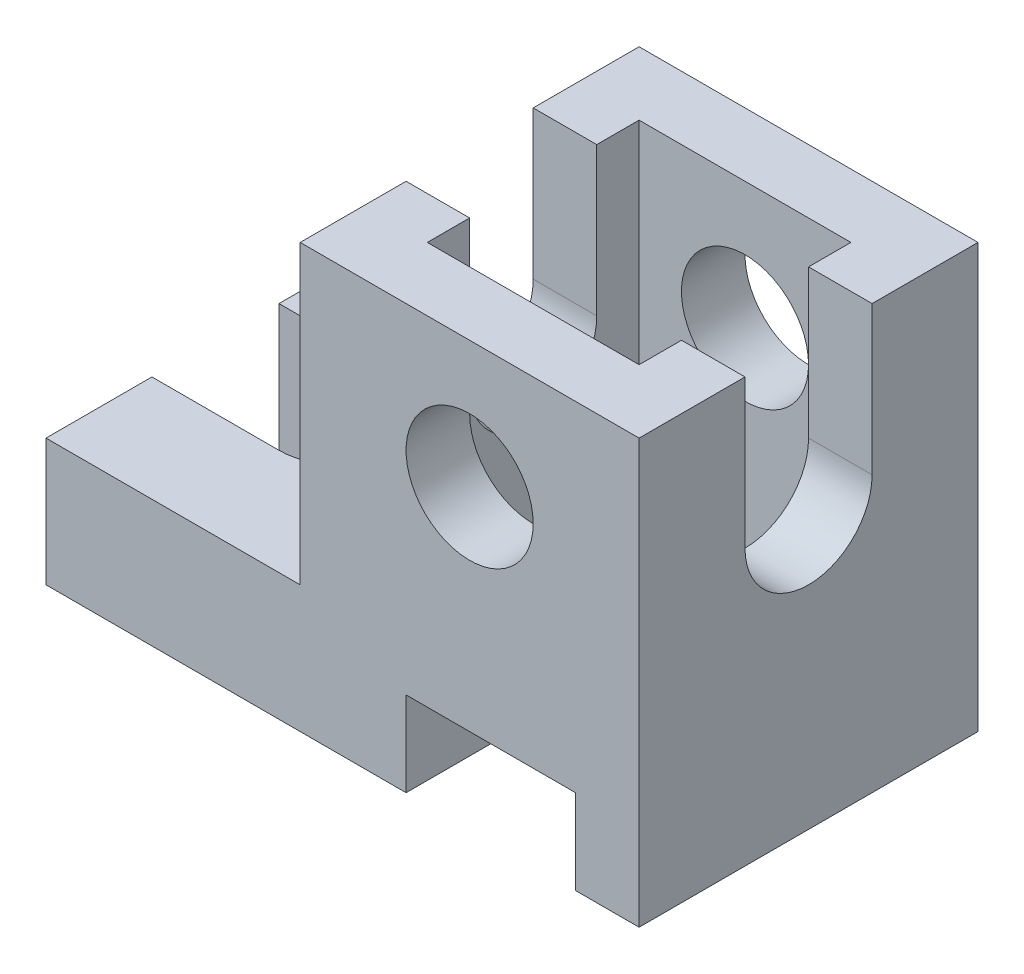
ISO-10303-21;
HEADER;
FILE_DESCRIPTION(('STEP AP214'),'2;1');
FILE_NAME('part.step','',(''),(''),'','','');
FILE_SCHEMA(('AUTOMOTIVE_DESIGN { 1 0 10303 214 1 1 1 1 }'));
ENDSEC;
DATA;
#1=APPLICATION_CONTEXT('core data for automotive mechanical design processes');
#2=APPLICATION_PROTOCOL_DEFINITION('international standard','automotive_design',2000,#1);
#3=PRODUCT_CONTEXT('',#1,'mechanical');
#4=PRODUCT('Part','Part','',(#3));
#5=PRODUCT_RELATED_PRODUCT_CATEGORY('part','',(#4));
#6=PRODUCT_DEFINITION_FORMATION('','',#4);
#7=PRODUCT_DEFINITION_CONTEXT('part definition',#1,'design');
#8=PRODUCT_DEFINITION('design','',#6,#7);
#9=PRODUCT_DEFINITION_SHAPE('','',#8);
#10=(LENGTH_UNIT() NAMED_UNIT(*) SI_UNIT(.MILLI.,.METRE.));
#11=(NAMED_UNIT(*) PLANE_ANGLE_UNIT() SI_UNIT($,.RADIAN.));
#12=(NAMED_UNIT(*) SI_UNIT($,.STERADIAN.) SOLID_ANGLE_UNIT());
#13=UNCERTAINTY_MEASURE_WITH_UNIT(LENGTH_MEASURE(1.E-05),#10,'distance_accuracy_value','');
#14=(GEOMETRIC_REPRESENTATION_CONTEXT(3) GLOBAL_UNCERTAINTY_ASSIGNED_CONTEXT((#13)) GLOBAL_UNIT_ASSIGNED_CONTEXT((#10,
#11,#12)) REPRESENTATION_CONTEXT('',''));
#15=CARTESIAN_POINT('',(0.,0.,0.));
#16=DIRECTION('',(0.,0.,1.));
#17=DIRECTION('',(1.,0.,0.));
#18=AXIS2_PLACEMENT_3D('',#15,#16,#17);
#19=CARTESIAN_POINT('',(140.,0.,-80.));
#20=DIRECTION('',(0.,-1.,0.));
#21=DIRECTION('',(0.,0.,-1.));
#22=AXIS2_PLACEMENT_3D('',#19,#20,#21);
#23=PLANE('',#22);
#24=DIRECTION('',(0.,0.,1.));
#25=VECTOR('',#24,1.);
#26=CARTESIAN_POINT('',(0.,0.,-80.));
#27=LINE('',#26,#25);
#28=CARTESIAN_POINT('',(0.,0.,-25.));
#29=VERTEX_POINT('',#28);
#30=CARTESIAN_POINT('',(0.,0.,0.));
#31=VERTEX_POINT('',#30);
#32=EDGE_CURVE('E244',#29,#31,#27,.T.);
#33=ORIENTED_EDGE('',*,*,#32,.F.);
#34=DIRECTION('',(1.,0.,0.));
#35=VECTOR('',#34,1.);
#36=CARTESIAN_POINT('',(140.,0.,-25.));
#37=LINE('',#36,#35);
#38=CARTESIAN_POINT('',(30.,0.,-25.));
#39=VERTEX_POINT('',#38);
#40=EDGE_CURVE('E285',#29,#39,#37,.T.);
#41=ORIENTED_EDGE('',*,*,#40,.T.);
#42=CARTESIAN_POINT('',(30.,0.,-40.));
#43=DIRECTION('',(0.,-1.,0.));
#44=DIRECTION('',(0.,0.,-1.));
#45=AXIS2_PLACEMENT_3D('',#42,#43,#44);
#46=CIRCLE('',#45,15.);
#47=CARTESIAN_POINT('',(30.,0.,-55.));
#48=VERTEX_POINT('',#47);
#49=EDGE_CURVE('E272',#39,#48,#46,.F.);
#50=ORIENTED_EDGE('',*,*,#49,.T.);
#51=DIRECTION('',(-1.,0.,0.));
#52=VECTOR('',#51,1.);
#53=CARTESIAN_POINT('',(140.,0.,-55.));
#54=LINE('',#53,#52);
#55=CARTESIAN_POINT('',(0.,0.,-55.));
#56=VERTEX_POINT('',#55);
#57=EDGE_CURVE('E277',#48,#56,#54,.T.);
#58=ORIENTED_EDGE('',*,*,#57,.T.);
#59=CARTESIAN_POINT('',(0.,0.,-80.));
#60=VERTEX_POINT('',#59);
#61=EDGE_CURVE('E239',#60,#56,#27,.T.);
#62=ORIENTED_EDGE('',*,*,#61,.F.);
#63=DIRECTION('',(1.,0.,0.));
#64=VECTOR('',#63,1.);
#65=CARTESIAN_POINT('',(140.,0.,-80.));
#66=LINE('',#65,#64);
#67=CARTESIAN_POINT('',(85.,0.,-80.));
#68=VERTEX_POINT('',#67);
#69=EDGE_CURVE('E420',#60,#68,#66,.T.);
#70=ORIENTED_EDGE('',*,*,#69,.T.);
#71=DIRECTION('',(0.,0.,1.));
#72=VECTOR('',#71,1.);
#73=CARTESIAN_POINT('',(85.,0.,-80.));
#74=LINE('',#73,#72);
#75=CARTESIAN_POINT('',(85.,0.,0.));
#76=VERTEX_POINT('',#75);
#77=EDGE_CURVE('E408',#68,#76,#74,.T.);
#78=ORIENTED_EDGE('',*,*,#77,.T.);
#79=DIRECTION('',(1.,0.,0.));
#80=VECTOR('',#79,1.);
#81=CARTESIAN_POINT('',(140.,0.,0.));
#82=LINE('',#81,#80);
#83=EDGE_CURVE('E430',#31,#76,#82,.T.);
#84=ORIENTED_EDGE('',*,*,#83,.F.);
#85=EDGE_LOOP('',(#33,#41,#50,#58,#62,#70,#78,#84));
#86=FACE_BOUND('',#85,.T.);
#87=ADVANCED_FACE('F44',(#86),#23,.T.);
#88=CARTESIAN_POINT('',(0.,0.,-80.));
#89=DIRECTION('',(-1.,0.,0.));
#90=DIRECTION('',(0.,0.,1.));
#91=AXIS2_PLACEMENT_3D('',#88,#89,#90);
#92=PLANE('',#91);
#93=DIRECTION('',(0.,0.,1.));
#94=VECTOR('',#93,1.);
#95=CARTESIAN_POINT('',(0.,30.,-80.));
#96=LINE('',#95,#94);
#97=CARTESIAN_POINT('',(0.,30.,-25.));
#98=VERTEX_POINT('',#97);
#99=CARTESIAN_POINT('',(0.,30.,0.));
#100=VERTEX_POINT('',#99);
#101=EDGE_CURVE('E247',#98,#100,#96,.T.);
#102=ORIENTED_EDGE('',*,*,#101,.F.);
#103=DIRECTION('',(0.,-1.,0.));
#104=VECTOR('',#103,1.);
#105=CARTESIAN_POINT('',(0.,40.,-25.));
#106=LINE('',#105,#104);
#107=EDGE_CURVE('E238',#98,#29,#106,.T.);
#108=ORIENTED_EDGE('',*,*,#107,.T.);
#109=ORIENTED_EDGE('',*,*,#32,.T.);
#110=DIRECTION('',(0.,-1.,0.));
#111=VECTOR('',#110,1.);
#112=CARTESIAN_POINT('',(0.,0.,0.));
#113=LINE('',#112,#111);
#114=EDGE_CURVE('E434',#100,#31,#113,.T.);
#115=ORIENTED_EDGE('',*,*,#114,.F.);
#116=EDGE_LOOP('',(#102,#108,#109,#115));
#117=FACE_BOUND('',#116,.T.);
#118=ADVANCED_FACE('F484',(#117),#92,.T.);
#119=ORIENTED_EDGE('',*,*,#61,.T.);
#120=DIRECTION('',(0.,-1.,0.));
#121=VECTOR('',#120,1.);
#122=CARTESIAN_POINT('',(0.,40.,-55.));
#123=LINE('',#122,#121);
#124=CARTESIAN_POINT('',(0.,30.,-55.));
#125=VERTEX_POINT('',#124);
#126=EDGE_CURVE('E223',#125,#56,#123,.T.);
#127=ORIENTED_EDGE('',*,*,#126,.F.);
#128=CARTESIAN_POINT('',(0.,30.,-80.));
#129=VERTEX_POINT('',#128);
#130=EDGE_CURVE('E240',#129,#125,#96,.T.);
#131=ORIENTED_EDGE('',*,*,#130,.F.);
#132=DIRECTION('',(0.,-1.,0.));
#133=VECTOR('',#132,1.);
#134=CARTESIAN_POINT('',(0.,0.,-80.));
#135=LINE('',#134,#133);
#136=EDGE_CURVE('E255',#129,#60,#135,.T.);
#137=ORIENTED_EDGE('',*,*,#136,.T.);
#138=EDGE_LOOP('',(#119,#127,#131,#137));
#139=FACE_BOUND('',#138,.T.);
#140=ADVANCED_FACE('F233',(#139),#92,.T.);
#141=CARTESIAN_POINT('',(0.,30.,-80.));
#142=DIRECTION('',(0.,1.,0.));
#143=DIRECTION('',(0.,0.,1.));
#144=AXIS2_PLACEMENT_3D('',#141,#142,#143);
#145=PLANE('',#144);
#146=CARTESIAN_POINT('',(30.,30.,-40.));
#147=DIRECTION('',(0.,1.,0.));
#148=DIRECTION('',(0.,0.,1.));
#149=AXIS2_PLACEMENT_3D('',#146,#147,#148);
#150=CIRCLE('',#149,15.);
#151=CARTESIAN_POINT('',(30.,30.,-55.));
#152=VERTEX_POINT('',#151);
#153=CARTESIAN_POINT('',(30.,30.,-25.));
#154=VERTEX_POINT('',#153);
#155=EDGE_CURVE('E52',#152,#154,#150,.F.);
#156=ORIENTED_EDGE('',*,*,#155,.T.);
#157=DIRECTION('',(-1.,0.,0.));
#158=VECTOR('',#157,1.);
#159=CARTESIAN_POINT('',(0.,30.,-25.));
#160=LINE('',#159,#158);
#161=EDGE_CURVE('E11',#154,#98,#160,.T.);
#162=ORIENTED_EDGE('',*,*,#161,.T.);
#163=ORIENTED_EDGE('',*,*,#101,.T.);
#164=DIRECTION('',(-1.,0.,0.));
#165=VECTOR('',#164,1.);
#166=CARTESIAN_POINT('',(0.,30.,0.));
#167=LINE('',#166,#165);
#168=CARTESIAN_POINT('',(60.,30.,0.));
#169=VERTEX_POINT('',#168);
#170=EDGE_CURVE('E433',#169,#100,#167,.T.);
#171=ORIENTED_EDGE('',*,*,#170,.F.);
#172=DIRECTION('',(0.,0.,1.));
#173=VECTOR('',#172,1.);
#174=CARTESIAN_POINT('',(60.,30.,-80.));
#175=LINE('',#174,#173);
#176=CARTESIAN_POINT('',(60.,30.,-80.));
#177=VERTEX_POINT('',#176);
#178=EDGE_CURVE('E378',#177,#169,#175,.T.);
#179=ORIENTED_EDGE('',*,*,#178,.F.);
#180=DIRECTION('',(-1.,0.,0.));
#181=VECTOR('',#180,1.);
#182=CARTESIAN_POINT('',(0.,30.,-80.));
#183=LINE('',#182,#181);
#184=EDGE_CURVE('E242',#177,#129,#183,.T.);
#185=ORIENTED_EDGE('',*,*,#184,.T.);
#186=ORIENTED_EDGE('',*,*,#130,.T.);
#187=DIRECTION('',(1.,0.,0.));
#188=VECTOR('',#187,1.);
#189=CARTESIAN_POINT('',(0.,30.,-55.));
#190=LINE('',#189,#188);
#191=EDGE_CURVE('E225',#125,#152,#190,.T.);
#192=ORIENTED_EDGE('',*,*,#191,.T.);
#193=EDGE_LOOP('',(#156,#162,#163,#171,#179,#185,#186,#192));
#194=FACE_BOUND('',#193,.T.);
#195=ADVANCED_FACE('F245',(#194),#145,.T.);
#196=CARTESIAN_POINT('',(140.,100.,-80.));
#197=DIRECTION('',(0.,1.,0.));
#198=DIRECTION('',(0.,0.,1.));
#199=AXIS2_PLACEMENT_3D('',#196,#197,#198);
#200=PLANE('',#199);
#201=DIRECTION('',(0.,0.,1.));
#202=VECTOR('',#201,1.);
#203=CARTESIAN_POINT('',(60.,100.,-80.));
#204=LINE('',#203,#202);
#205=CARTESIAN_POINT('',(60.,100.,-80.));
#206=VERTEX_POINT('',#205);
#207=CARTESIAN_POINT('',(60.,100.,-55.));
#208=VERTEX_POINT('',#207);
#209=EDGE_CURVE('E385',#206,#208,#204,.T.);
#210=ORIENTED_EDGE('',*,*,#209,.T.);
#211=DIRECTION('',(-1.,0.,0.));
#212=VECTOR('',#211,1.);
#213=CARTESIAN_POINT('',(140.,100.,-55.));
#214=LINE('',#213,#212);
#215=CARTESIAN_POINT('',(75.,100.,-55.));
#216=VERTEX_POINT('',#215);
#217=EDGE_CURVE('E301',#216,#208,#214,.T.);
#218=ORIENTED_EDGE('',*,*,#217,.F.);
#219=DIRECTION('',(0.,0.,-1.));
#220=VECTOR('',#219,1.);
#221=CARTESIAN_POINT('',(75.,100.,0.));
#222=LINE('',#221,#220);
#223=CARTESIAN_POINT('',(75.,100.,-65.));
#224=VERTEX_POINT('',#223);
#225=EDGE_CURVE('E330',#216,#224,#222,.T.);
#226=ORIENTED_EDGE('',*,*,#225,.T.);
#227=DIRECTION('',(1.,0.,0.));
#228=VECTOR('',#227,1.);
#229=CARTESIAN_POINT('',(0.,100.,-65.));
#230=LINE('',#229,#228);
#231=CARTESIAN_POINT('',(125.,100.,-65.));
#232=VERTEX_POINT('',#231);
#233=EDGE_CURVE('E335',#224,#232,#230,.T.);
#234=ORIENTED_EDGE('',*,*,#233,.T.);
#235=DIRECTION('',(0.,0.,1.));
#236=VECTOR('',#235,1.);
#237=CARTESIAN_POINT('',(125.,100.,0.));
#238=LINE('',#237,#236);
#239=CARTESIAN_POINT('',(125.,100.,-55.));
#240=VERTEX_POINT('',#239);
#241=EDGE_CURVE('E346',#232,#240,#238,.T.);
#242=ORIENTED_EDGE('',*,*,#241,.T.);
#243=CARTESIAN_POINT('',(140.,100.,-55.));
#244=VERTEX_POINT('',#243);
#245=EDGE_CURVE('E302',#244,#240,#214,.T.);
#246=ORIENTED_EDGE('',*,*,#245,.F.);
#247=DIRECTION('',(0.,0.,1.));
#248=VECTOR('',#247,1.);
#249=CARTESIAN_POINT('',(140.,100.,-80.));
#250=LINE('',#249,#248);
#251=CARTESIAN_POINT('',(140.,100.,-80.));
#252=VERTEX_POINT('',#251);
#253=EDGE_CURVE('E387',#252,#244,#250,.T.);
#254=ORIENTED_EDGE('',*,*,#253,.F.);
#255=DIRECTION('',(-1.,0.,0.));
#256=VECTOR('',#255,1.);
#257=CARTESIAN_POINT('',(140.,100.,-80.));
#258=LINE('',#257,#256);
#259=EDGE_CURVE('E368',#252,#206,#258,.T.);
#260=ORIENTED_EDGE('',*,*,#259,.T.);
#261=EDGE_LOOP('',(#210,#218,#226,#234,#242,#246,#254,#260));
#262=FACE_BOUND('',#261,.T.);
#263=ADVANCED_FACE('F451',(#262),#200,.T.);
#264=CARTESIAN_POINT('',(140.,100.,-25.));
#265=VERTEX_POINT('',#264);
#266=CARTESIAN_POINT('',(140.,100.,0.));
#267=VERTEX_POINT('',#266);
#268=EDGE_CURVE('E373',#265,#267,#250,.T.);
#269=ORIENTED_EDGE('',*,*,#268,.F.);
#270=DIRECTION('',(-1.,0.,0.));
#271=VECTOR('',#270,1.);
#272=CARTESIAN_POINT('',(140.,100.,-25.));
#273=LINE('',#272,#271);
#274=CARTESIAN_POINT('',(125.,100.,-25.));
#275=VERTEX_POINT('',#274);
#276=EDGE_CURVE('E303',#265,#275,#273,.T.);
#277=ORIENTED_EDGE('',*,*,#276,.T.);
#278=CARTESIAN_POINT('',(125.,100.,-15.));
#279=VERTEX_POINT('',#278);
#280=EDGE_CURVE('E350',#275,#279,#238,.T.);
#281=ORIENTED_EDGE('',*,*,#280,.T.);
#282=DIRECTION('',(-1.,0.,0.));
#283=VECTOR('',#282,1.);
#284=CARTESIAN_POINT('',(0.,100.,-15.));
#285=LINE('',#284,#283);
#286=CARTESIAN_POINT('',(75.,100.,-15.));
#287=VERTEX_POINT('',#286);
#288=EDGE_CURVE('E341',#279,#287,#285,.T.);
#289=ORIENTED_EDGE('',*,*,#288,.T.);
#290=CARTESIAN_POINT('',(75.,100.,-25.));
#291=VERTEX_POINT('',#290);
#292=EDGE_CURVE('E342',#287,#291,#222,.T.);
#293=ORIENTED_EDGE('',*,*,#292,.T.);
#294=CARTESIAN_POINT('',(60.,100.,-25.));
#295=VERTEX_POINT('',#294);
#296=EDGE_CURVE('E306',#291,#295,#273,.T.);
#297=ORIENTED_EDGE('',*,*,#296,.T.);
#298=CARTESIAN_POINT('',(60.,100.,0.));
#299=VERTEX_POINT('',#298);
#300=EDGE_CURVE('E384',#295,#299,#204,.T.);
#301=ORIENTED_EDGE('',*,*,#300,.T.);
#302=DIRECTION('',(-1.,0.,0.));
#303=VECTOR('',#302,1.);
#304=CARTESIAN_POINT('',(140.,100.,0.));
#305=LINE('',#304,#303);
#306=EDGE_CURVE('E364',#267,#299,#305,.T.);
#307=ORIENTED_EDGE('',*,*,#306,.F.);
#308=EDGE_LOOP('',(#269,#277,#281,#289,#293,#297,#301,#307));
#309=FACE_BOUND('',#308,.T.);
#310=ADVANCED_FACE('F475',(#309),#200,.T.);
#311=CARTESIAN_POINT('',(140.,30.,-80.));
#312=DIRECTION('',(1.,0.,0.));
#313=DIRECTION('',(0.,0.,-1.));
#314=AXIS2_PLACEMENT_3D('',#311,#312,#313);
#315=PLANE('',#314);
#316=ORIENTED_EDGE('',*,*,#253,.T.);
#317=DIRECTION('',(0.,1.,0.));
#318=VECTOR('',#317,1.);
#319=CARTESIAN_POINT('',(140.,0.,-55.));
#320=LINE('',#319,#318);
#321=CARTESIAN_POINT('',(140.,65.,-55.));
#322=VERTEX_POINT('',#321);
#323=EDGE_CURVE('E284',#322,#244,#320,.T.);
#324=ORIENTED_EDGE('',*,*,#323,.F.);
#325=CARTESIAN_POINT('',(140.,65.,-40.));
#326=DIRECTION('',(-1.,0.,0.));
#327=DIRECTION('',(0.,0.,1.));
#328=AXIS2_PLACEMENT_3D('',#325,#326,#327);
#329=CIRCLE('',#328,15.);
#330=CARTESIAN_POINT('',(140.,65.,-25.));
#331=VERTEX_POINT('',#330);
#332=EDGE_CURVE('E289',#322,#331,#329,.T.);
#333=ORIENTED_EDGE('',*,*,#332,.T.);
#334=DIRECTION('',(0.,-1.,0.));
#335=VECTOR('',#334,1.);
#336=CARTESIAN_POINT('',(140.,0.,-25.));
#337=LINE('',#336,#335);
#338=EDGE_CURVE('E292',#265,#331,#337,.T.);
#339=ORIENTED_EDGE('',*,*,#338,.F.);
#340=ORIENTED_EDGE('',*,*,#268,.T.);
#341=DIRECTION('',(0.,1.,0.));
#342=VECTOR('',#341,1.);
#343=CARTESIAN_POINT('',(140.,30.,0.));
#344=LINE('',#343,#342);
#345=CARTESIAN_POINT('',(140.,0.,0.));
#346=VERTEX_POINT('',#345);
#347=EDGE_CURVE('E429',#346,#267,#344,.T.);
#348=ORIENTED_EDGE('',*,*,#347,.F.);
#349=DIRECTION('',(0.,0.,1.));
#350=VECTOR('',#349,1.);
#351=CARTESIAN_POINT('',(140.,0.,-80.));
#352=LINE('',#351,#350);
#353=CARTESIAN_POINT('',(140.,0.,-80.));
#354=VERTEX_POINT('',#353);
#355=EDGE_CURVE('E246',#354,#346,#352,.T.);
#356=ORIENTED_EDGE('',*,*,#355,.F.);
#357=DIRECTION('',(0.,1.,0.));
#358=VECTOR('',#357,1.);
#359=CARTESIAN_POINT('',(140.,30.,-80.));
#360=LINE('',#359,#358);
#361=EDGE_CURVE('E425',#354,#252,#360,.T.);
#362=ORIENTED_EDGE('',*,*,#361,.T.);
#363=EDGE_LOOP('',(#316,#324,#333,#339,#340,#348,#356,#362));
#364=FACE_BOUND('',#363,.T.);
#365=ADVANCED_FACE('F446',(#364),#315,.T.);
#366=CARTESIAN_POINT('',(125.,0.,-80.));
#367=DIRECTION('',(1.,0.,0.));
#368=DIRECTION('',(0.,0.,-1.));
#369=AXIS2_PLACEMENT_3D('',#366,#367,#368);
#370=PLANE('',#369);
#371=DIRECTION('',(0.,-1.,0.));
#372=VECTOR('',#371,1.);
#373=CARTESIAN_POINT('',(125.,0.,-55.));
#374=LINE('',#373,#372);
#375=CARTESIAN_POINT('',(125.,65.,-55.));
#376=VERTEX_POINT('',#375);
#377=EDGE_CURVE('E318',#240,#376,#374,.T.);
#378=ORIENTED_EDGE('',*,*,#377,.F.);
#379=ORIENTED_EDGE('',*,*,#241,.F.);
#380=DIRECTION('',(0.,1.,0.));
#381=VECTOR('',#380,1.);
#382=CARTESIAN_POINT('',(125.,20.,-65.));
#383=LINE('',#382,#381);
#384=CARTESIAN_POINT('',(125.,20.,-65.));
#385=VERTEX_POINT('',#384);
#386=EDGE_CURVE('E359',#385,#232,#383,.T.);
#387=ORIENTED_EDGE('',*,*,#386,.F.);
#388=DIRECTION('',(0.,0.,1.));
#389=VECTOR('',#388,1.);
#390=CARTESIAN_POINT('',(125.,20.,-80.));
#391=LINE('',#390,#389);
#392=CARTESIAN_POINT('',(125.,20.,-80.));
#393=VERTEX_POINT('',#392);
#394=EDGE_CURVE('E411',#393,#385,#391,.T.);
#395=ORIENTED_EDGE('',*,*,#394,.F.);
#396=DIRECTION('',(0.,1.,0.));
#397=VECTOR('',#396,1.);
#398=CARTESIAN_POINT('',(125.,0.,-80.));
#399=LINE('',#398,#397);
#400=CARTESIAN_POINT('',(125.,0.,-80.));
#401=VERTEX_POINT('',#400);
#402=EDGE_CURVE('E386',#401,#393,#399,.T.);
#403=ORIENTED_EDGE('',*,*,#402,.F.);
#404=DIRECTION('',(0.,0.,1.));
#405=VECTOR('',#404,1.);
#406=CARTESIAN_POINT('',(125.,0.,-80.));
#407=LINE('',#406,#405);
#408=CARTESIAN_POINT('',(125.,0.,0.));
#409=VERTEX_POINT('',#408);
#410=EDGE_CURVE('E396',#401,#409,#407,.T.);
#411=ORIENTED_EDGE('',*,*,#410,.T.);
#412=DIRECTION('',(0.,1.,0.));
#413=VECTOR('',#412,1.);
#414=CARTESIAN_POINT('',(125.,0.,0.));
#415=LINE('',#414,#413);
#416=CARTESIAN_POINT('',(125.,20.,0.));
#417=VERTEX_POINT('',#416);
#418=EDGE_CURVE('E381',#409,#417,#415,.T.);
#419=ORIENTED_EDGE('',*,*,#418,.T.);
#420=CARTESIAN_POINT('',(125.,20.,-15.));
#421=VERTEX_POINT('',#420);
#422=EDGE_CURVE('E417',#421,#417,#391,.T.);
#423=ORIENTED_EDGE('',*,*,#422,.F.);
#424=DIRECTION('',(0.,1.,0.));
#425=VECTOR('',#424,1.);
#426=CARTESIAN_POINT('',(125.,20.,-15.));
#427=LINE('',#426,#425);
#428=EDGE_CURVE('E356',#421,#279,#427,.T.);
#429=ORIENTED_EDGE('',*,*,#428,.T.);
#430=ORIENTED_EDGE('',*,*,#280,.F.);
#431=DIRECTION('',(0.,1.,0.));
#432=VECTOR('',#431,1.);
#433=CARTESIAN_POINT('',(125.,0.,-25.));
#434=LINE('',#433,#432);
#435=CARTESIAN_POINT('',(125.,65.,-25.));
#436=VERTEX_POINT('',#435);
#437=EDGE_CURVE('E316',#436,#275,#434,.T.);
#438=ORIENTED_EDGE('',*,*,#437,.F.);
#439=CARTESIAN_POINT('',(125.,65.,-40.));
#440=DIRECTION('',(1.,0.,0.));
#441=DIRECTION('',(0.,0.,-1.));
#442=AXIS2_PLACEMENT_3D('',#439,#440,#441);
#443=CIRCLE('',#442,15.);
#444=EDGE_CURVE('E305',#436,#376,#443,.T.);
#445=ORIENTED_EDGE('',*,*,#444,.T.);
#446=EDGE_LOOP('',(#378,#379,#387,#395,#403,#411,#419,#423,#429,#430,#438,#445));
#447=FACE_BOUND('',#446,.T.);
#448=ADVANCED_FACE('F466',(#447),#370,.F.);
#449=CARTESIAN_POINT('',(60.,100.,-80.));
#450=DIRECTION('',(-1.,0.,0.));
#451=DIRECTION('',(0.,0.,1.));
#452=AXIS2_PLACEMENT_3D('',#449,#450,#451);
#453=PLANE('',#452);
#454=CARTESIAN_POINT('',(60.,65.,-40.));
#455=DIRECTION('',(-1.,0.,0.));
#456=DIRECTION('',(0.,0.,1.));
#457=AXIS2_PLACEMENT_3D('',#454,#455,#456);
#458=CIRCLE('',#457,15.);
#459=CARTESIAN_POINT('',(60.,65.,-55.));
#460=VERTEX_POINT('',#459);
#461=CARTESIAN_POINT('',(60.,65.,-25.));
#462=VERTEX_POINT('',#461);
#463=EDGE_CURVE('E298',#460,#462,#458,.T.);
#464=ORIENTED_EDGE('',*,*,#463,.F.);
#465=DIRECTION('',(0.,1.,0.));
#466=VECTOR('',#465,1.);
#467=CARTESIAN_POINT('',(60.,0.,-55.));
#468=LINE('',#467,#466);
#469=EDGE_CURVE('E282',#460,#208,#468,.T.);
#470=ORIENTED_EDGE('',*,*,#469,.T.);
#471=ORIENTED_EDGE('',*,*,#209,.F.);
#472=DIRECTION('',(0.,-1.,0.));
#473=VECTOR('',#472,1.);
#474=CARTESIAN_POINT('',(60.,100.,-80.));
#475=LINE('',#474,#473);
#476=EDGE_CURVE('E369',#206,#177,#475,.T.);
#477=ORIENTED_EDGE('',*,*,#476,.T.);
#478=ORIENTED_EDGE('',*,*,#178,.T.);
#479=DIRECTION('',(0.,-1.,0.));
#480=VECTOR('',#479,1.);
#481=CARTESIAN_POINT('',(60.,100.,0.));
#482=LINE('',#481,#480);
#483=EDGE_CURVE('E367',#299,#169,#482,.T.);
#484=ORIENTED_EDGE('',*,*,#483,.F.);
#485=ORIENTED_EDGE('',*,*,#300,.F.);
#486=DIRECTION('',(0.,-1.,0.));
#487=VECTOR('',#486,1.);
#488=CARTESIAN_POINT('',(60.,0.,-25.));
#489=LINE('',#488,#487);
#490=EDGE_CURVE('E290',#295,#462,#489,.T.);
#491=ORIENTED_EDGE('',*,*,#490,.T.);
#492=EDGE_LOOP('',(#464,#470,#471,#477,#478,#484,#485,#491));
#493=FACE_BOUND('',#492,.T.);
#494=ADVANCED_FACE('F483',(#493),#453,.T.);
#495=CARTESIAN_POINT('',(75.,20.,0.));
#496=DIRECTION('',(1.,0.,0.));
#497=DIRECTION('',(0.,0.,-1.));
#498=AXIS2_PLACEMENT_3D('',#495,#496,#497);
#499=PLANE('',#498);
#500=ORIENTED_EDGE('',*,*,#225,.F.);
#501=DIRECTION('',(0.,-1.,0.));
#502=VECTOR('',#501,1.);
#503=CARTESIAN_POINT('',(75.,20.,-55.));
#504=LINE('',#503,#502);
#505=CARTESIAN_POINT('',(75.,65.,-55.));
#506=VERTEX_POINT('',#505);
#507=EDGE_CURVE('E229',#216,#506,#504,.T.);
#508=ORIENTED_EDGE('',*,*,#507,.T.);
#509=CARTESIAN_POINT('',(75.,65.,-40.));
#510=DIRECTION('',(1.,0.,0.));
#511=DIRECTION('',(0.,0.,-1.));
#512=AXIS2_PLACEMENT_3D('',#509,#510,#511);
#513=CIRCLE('',#512,15.);
#514=CARTESIAN_POINT('',(75.,65.,-25.));
#515=VERTEX_POINT('',#514);
#516=EDGE_CURVE('E257',#515,#506,#513,.T.);
#517=ORIENTED_EDGE('',*,*,#516,.F.);
#518=DIRECTION('',(0.,1.,0.));
#519=VECTOR('',#518,1.);
#520=CARTESIAN_POINT('',(75.,20.,-25.));
#521=LINE('',#520,#519);
#522=EDGE_CURVE('E265',#515,#291,#521,.T.);
#523=ORIENTED_EDGE('',*,*,#522,.T.);
#524=ORIENTED_EDGE('',*,*,#292,.F.);
#525=DIRECTION('',(0.,1.,0.));
#526=VECTOR('',#525,1.);
#527=CARTESIAN_POINT('',(75.,20.,-15.));
#528=LINE('',#527,#526);
#529=CARTESIAN_POINT('',(75.,20.,-15.));
#530=VERTEX_POINT('',#529);
#531=EDGE_CURVE('E339',#530,#287,#528,.T.);
#532=ORIENTED_EDGE('',*,*,#531,.F.);
#533=DIRECTION('',(0.,0.,-1.));
#534=VECTOR('',#533,1.);
#535=CARTESIAN_POINT('',(75.,20.,0.));
#536=LINE('',#535,#534);
#537=CARTESIAN_POINT('',(75.,20.,-65.));
#538=VERTEX_POINT('',#537);
#539=EDGE_CURVE('E327',#530,#538,#536,.T.);
#540=ORIENTED_EDGE('',*,*,#539,.T.);
#541=DIRECTION('',(0.,1.,0.));
#542=VECTOR('',#541,1.);
#543=CARTESIAN_POINT('',(75.,20.,-65.));
#544=LINE('',#543,#542);
#545=EDGE_CURVE('E351',#538,#224,#544,.T.);
#546=ORIENTED_EDGE('',*,*,#545,.T.);
#547=EDGE_LOOP('',(#500,#508,#517,#523,#524,#532,#540,#546));
#548=FACE_BOUND('',#547,.T.);
#549=ADVANCED_FACE('F520',(#548),#499,.T.);
#550=CARTESIAN_POINT('',(0.,20.,-80.));
#551=DIRECTION('',(0.,1.,0.));
#552=DIRECTION('',(0.,0.,1.));
#553=AXIS2_PLACEMENT_3D('',#550,#551,#552);
#554=PLANE('',#553);
#555=DIRECTION('',(1.,0.,0.));
#556=VECTOR('',#555,1.);
#557=CARTESIAN_POINT('',(0.,20.,-65.));
#558=LINE('',#557,#556);
#559=CARTESIAN_POINT('',(85.,20.,-65.));
#560=VERTEX_POINT('',#559);
#561=EDGE_CURVE('E338',#560,#385,#558,.T.);
#562=ORIENTED_EDGE('',*,*,#561,.F.);
#563=DIRECTION('',(0.,0.,1.));
#564=VECTOR('',#563,1.);
#565=CARTESIAN_POINT('',(85.,20.,-80.));
#566=LINE('',#565,#564);
#567=CARTESIAN_POINT('',(85.,20.,-80.));
#568=VERTEX_POINT('',#567);
#569=EDGE_CURVE('E409',#568,#560,#566,.T.);
#570=ORIENTED_EDGE('',*,*,#569,.F.);
#571=DIRECTION('',(-1.,0.,0.));
#572=VECTOR('',#571,1.);
#573=CARTESIAN_POINT('',(0.,20.,-80.));
#574=LINE('',#573,#572);
#575=EDGE_CURVE('E395',#393,#568,#574,.T.);
#576=ORIENTED_EDGE('',*,*,#575,.F.);
#577=ORIENTED_EDGE('',*,*,#394,.T.);
#578=EDGE_LOOP('',(#562,#570,#576,#577));
#579=FACE_BOUND('',#578,.T.);
#580=ADVANCED_FACE('F502',(#579),#554,.F.);
#581=DIRECTION('',(-1.,0.,0.));
#582=VECTOR('',#581,1.);
#583=CARTESIAN_POINT('',(0.,20.,-15.));
#584=LINE('',#583,#582);
#585=CARTESIAN_POINT('',(85.,20.,-15.));
#586=VERTEX_POINT('',#585);
#587=EDGE_CURVE('E334',#421,#586,#584,.T.);
#588=ORIENTED_EDGE('',*,*,#587,.F.);
#589=ORIENTED_EDGE('',*,*,#422,.T.);
#590=DIRECTION('',(-1.,0.,0.));
#591=VECTOR('',#590,1.);
#592=CARTESIAN_POINT('',(0.,20.,0.));
#593=LINE('',#592,#591);
#594=CARTESIAN_POINT('',(85.,20.,0.));
#595=VERTEX_POINT('',#594);
#596=EDGE_CURVE('E405',#417,#595,#593,.T.);
#597=ORIENTED_EDGE('',*,*,#596,.T.);
#598=EDGE_CURVE('E415',#586,#595,#566,.T.);
#599=ORIENTED_EDGE('',*,*,#598,.F.);
#600=EDGE_LOOP('',(#588,#589,#597,#599));
#601=FACE_BOUND('',#600,.T.);
#602=ADVANCED_FACE('F496',(#601),#554,.F.);
#603=ORIENTED_EDGE('',*,*,#410,.F.);
#604=EDGE_CURVE('E421',#401,#354,#66,.T.);
#605=ORIENTED_EDGE('',*,*,#604,.T.);
#606=ORIENTED_EDGE('',*,*,#355,.T.);
#607=EDGE_CURVE('E407',#409,#346,#82,.T.);
#608=ORIENTED_EDGE('',*,*,#607,.F.);
#609=EDGE_LOOP('',(#603,#605,#606,#608));
#610=FACE_BOUND('',#609,.T.);
#611=ADVANCED_FACE('F50',(#610),#23,.T.);
#612=CARTESIAN_POINT('',(0.,0.,-80.));
#613=DIRECTION('',(0.,0.,-1.));
#614=DIRECTION('',(-1.,0.,0.));
#615=AXIS2_PLACEMENT_3D('',#612,#613,#614);
#616=PLANE('',#615);
#617=CARTESIAN_POINT('',(100.,70.,-80.));
#618=DIRECTION('',(0.,0.,1.));
#619=DIRECTION('',(1.,0.,0.));
#620=AXIS2_PLACEMENT_3D('',#617,#618,#619);
#621=CIRCLE('',#620,15.);
#622=CARTESIAN_POINT('',(115.,70.,-80.));
#623=VERTEX_POINT('',#622);
#624=EDGE_CURVE('E259',#623,#623,#621,.T.);
#625=ORIENTED_EDGE('',*,*,#624,.T.);
#626=EDGE_LOOP('',(#625));
#627=FACE_BOUND('',#626,.T.);
#628=DIRECTION('',(0.,-1.,0.));
#629=VECTOR('',#628,1.);
#630=CARTESIAN_POINT('',(85.,0.,-80.));
#631=LINE('',#630,#629);
#632=EDGE_CURVE('E397',#568,#68,#631,.T.);
#633=ORIENTED_EDGE('',*,*,#632,.T.);
#634=ORIENTED_EDGE('',*,*,#69,.F.);
#635=ORIENTED_EDGE('',*,*,#136,.F.);
#636=ORIENTED_EDGE('',*,*,#184,.F.);
#637=ORIENTED_EDGE('',*,*,#476,.F.);
#638=ORIENTED_EDGE('',*,*,#259,.F.);
#639=ORIENTED_EDGE('',*,*,#361,.F.);
#640=ORIENTED_EDGE('',*,*,#604,.F.);
#641=ORIENTED_EDGE('',*,*,#402,.T.);
#642=ORIENTED_EDGE('',*,*,#575,.T.);
#643=EDGE_LOOP('',(#633,#634,#635,#636,#637,#638,#639,#640,#641,#642));
#644=FACE_BOUND('',#643,.T.);
#645=ADVANCED_FACE('F452',(#627,#644),#616,.T.);
#646=CARTESIAN_POINT('',(0.,0.,0.));
#647=DIRECTION('',(0.,0.,-1.));
#648=DIRECTION('',(-1.,0.,0.));
#649=AXIS2_PLACEMENT_3D('',#646,#647,#648);
#650=PLANE('',#649);
#651=CARTESIAN_POINT('',(100.,70.,0.));
#652=DIRECTION('',(0.,0.,1.));
#653=DIRECTION('',(1.,0.,0.));
#654=AXIS2_PLACEMENT_3D('',#651,#652,#653);
#655=CIRCLE('',#654,15.);
#656=CARTESIAN_POINT('',(115.,70.,0.));
#657=VERTEX_POINT('',#656);
#658=EDGE_CURVE('E319',#657,#657,#655,.T.);
#659=ORIENTED_EDGE('',*,*,#658,.F.);
#660=EDGE_LOOP('',(#659));
#661=FACE_BOUND('',#660,.T.);
#662=ORIENTED_EDGE('',*,*,#83,.T.);
#663=DIRECTION('',(0.,-1.,0.));
#664=VECTOR('',#663,1.);
#665=CARTESIAN_POINT('',(85.,0.,0.));
#666=LINE('',#665,#664);
#667=EDGE_CURVE('E391',#595,#76,#666,.T.);
#668=ORIENTED_EDGE('',*,*,#667,.F.);
#669=ORIENTED_EDGE('',*,*,#596,.F.);
#670=ORIENTED_EDGE('',*,*,#418,.F.);
#671=ORIENTED_EDGE('',*,*,#607,.T.);
#672=ORIENTED_EDGE('',*,*,#347,.T.);
#673=ORIENTED_EDGE('',*,*,#306,.T.);
#674=ORIENTED_EDGE('',*,*,#483,.T.);
#675=ORIENTED_EDGE('',*,*,#170,.T.);
#676=ORIENTED_EDGE('',*,*,#114,.T.);
#677=EDGE_LOOP('',(#662,#668,#669,#670,#671,#672,#673,#674,#675,#676));
#678=FACE_BOUND('',#677,.T.);
#679=ADVANCED_FACE('F478',(#661,#678),#650,.F.);
#680=CARTESIAN_POINT('',(85.,0.,-80.));
#681=DIRECTION('',(-1.,0.,0.));
#682=DIRECTION('',(0.,0.,1.));
#683=AXIS2_PLACEMENT_3D('',#680,#681,#682);
#684=PLANE('',#683);
#685=ORIENTED_EDGE('',*,*,#667,.T.);
#686=ORIENTED_EDGE('',*,*,#77,.F.);
#687=ORIENTED_EDGE('',*,*,#632,.F.);
#688=ORIENTED_EDGE('',*,*,#569,.T.);
#689=DIRECTION('',(0.,0.,-1.));
#690=VECTOR('',#689,1.);
#691=CARTESIAN_POINT('',(85.,20.,-80.));
#692=LINE('',#691,#690);
#693=EDGE_CURVE('E357',#586,#560,#692,.T.);
#694=ORIENTED_EDGE('',*,*,#693,.F.);
#695=ORIENTED_EDGE('',*,*,#598,.T.);
#696=EDGE_LOOP('',(#685,#686,#687,#688,#694,#695));
#697=FACE_BOUND('',#696,.T.);
#698=ADVANCED_FACE('F492',(#697),#684,.F.);
#699=CARTESIAN_POINT('',(0.,20.,0.));
#700=DIRECTION('',(0.,1.,0.));
#701=DIRECTION('',(0.,0.,1.));
#702=AXIS2_PLACEMENT_3D('',#699,#700,#701);
#703=PLANE('',#702);
#704=ORIENTED_EDGE('',*,*,#693,.T.);
#705=EDGE_CURVE('E340',#538,#560,#558,.T.);
#706=ORIENTED_EDGE('',*,*,#705,.F.);
#707=ORIENTED_EDGE('',*,*,#539,.F.);
#708=EDGE_CURVE('E332',#586,#530,#584,.T.);
#709=ORIENTED_EDGE('',*,*,#708,.F.);
#710=EDGE_LOOP('',(#704,#706,#707,#709));
#711=FACE_BOUND('',#710,.T.);
#712=ADVANCED_FACE('F511',(#711),#703,.T.);
#713=CARTESIAN_POINT('',(0.,20.,-65.));
#714=DIRECTION('',(0.,0.,1.));
#715=DIRECTION('',(1.,0.,0.));
#716=AXIS2_PLACEMENT_3D('',#713,#714,#715);
#717=PLANE('',#716);
#718=CARTESIAN_POINT('',(100.,70.,-65.));
#719=DIRECTION('',(0.,0.,1.));
#720=DIRECTION('',(1.,0.,0.));
#721=AXIS2_PLACEMENT_3D('',#718,#719,#720);
#722=CIRCLE('',#721,15.);
#723=CARTESIAN_POINT('',(115.,70.,-65.));
#724=VERTEX_POINT('',#723);
#725=EDGE_CURVE('E256',#724,#724,#722,.T.);
#726=ORIENTED_EDGE('',*,*,#725,.F.);
#727=EDGE_LOOP('',(#726));
#728=FACE_BOUND('',#727,.T.);
#729=ORIENTED_EDGE('',*,*,#233,.F.);
#730=ORIENTED_EDGE('',*,*,#545,.F.);
#731=ORIENTED_EDGE('',*,*,#705,.T.);
#732=ORIENTED_EDGE('',*,*,#561,.T.);
#733=ORIENTED_EDGE('',*,*,#386,.T.);
#734=EDGE_LOOP('',(#729,#730,#731,#732,#733));
#735=FACE_BOUND('',#734,.T.);
#736=ADVANCED_FACE('F510',(#728,#735),#717,.T.);
#737=CARTESIAN_POINT('',(0.,20.,-15.));
#738=DIRECTION('',(0.,0.,-1.));
#739=DIRECTION('',(-1.,0.,0.));
#740=AXIS2_PLACEMENT_3D('',#737,#738,#739);
#741=PLANE('',#740);
#742=CARTESIAN_POINT('',(100.,70.,-15.));
#743=DIRECTION('',(0.,0.,-1.));
#744=DIRECTION('',(-1.,0.,0.));
#745=AXIS2_PLACEMENT_3D('',#742,#743,#744);
#746=CIRCLE('',#745,15.);
#747=CARTESIAN_POINT('',(85.,70.,-15.));
#748=VERTEX_POINT('',#747);
#749=EDGE_CURVE('E254',#748,#748,#746,.T.);
#750=ORIENTED_EDGE('',*,*,#749,.F.);
#751=EDGE_LOOP('',(#750));
#752=FACE_BOUND('',#751,.T.);
#753=ORIENTED_EDGE('',*,*,#288,.F.);
#754=ORIENTED_EDGE('',*,*,#428,.F.);
#755=ORIENTED_EDGE('',*,*,#587,.T.);
#756=ORIENTED_EDGE('',*,*,#708,.T.);
#757=ORIENTED_EDGE('',*,*,#531,.T.);
#758=EDGE_LOOP('',(#753,#754,#755,#756,#757));
#759=FACE_BOUND('',#758,.T.);
#760=ADVANCED_FACE('F517',(#752,#759),#741,.T.);
#761=CARTESIAN_POINT('',(100.,70.,-80.));
#762=DIRECTION('',(0.,0.,1.));
#763=DIRECTION('',(1.,0.,0.));
#764=AXIS2_PLACEMENT_3D('',#761,#762,#763);
#765=CYLINDRICAL_SURFACE('',#764,15.);
#766=ORIENTED_EDGE('',*,*,#749,.T.);
#767=EDGE_LOOP('',(#766));
#768=FACE_BOUND('',#767,.T.);
#769=ORIENTED_EDGE('',*,*,#658,.T.);
#770=EDGE_LOOP('',(#769));
#771=FACE_BOUND('',#770,.T.);
#772=ADVANCED_FACE('F522',(#768,#771),#765,.F.);
#773=ORIENTED_EDGE('',*,*,#725,.T.);
#774=EDGE_LOOP('',(#773));
#775=FACE_BOUND('',#774,.T.);
#776=ORIENTED_EDGE('',*,*,#624,.F.);
#777=EDGE_LOOP('',(#776));
#778=FACE_BOUND('',#777,.T.);
#779=ADVANCED_FACE('F530',(#775,#778),#765,.F.);
#780=CARTESIAN_POINT('',(140.,65.,-40.));
#781=DIRECTION('',(-1.,0.,0.));
#782=DIRECTION('',(0.,0.,1.));
#783=AXIS2_PLACEMENT_3D('',#780,#781,#782);
#784=CYLINDRICAL_SURFACE('',#783,15.);
#785=ORIENTED_EDGE('',*,*,#516,.T.);
#786=DIRECTION('',(-1.,0.,0.));
#787=VECTOR('',#786,1.);
#788=CARTESIAN_POINT('',(140.,65.,-55.));
#789=LINE('',#788,#787);
#790=EDGE_CURVE('E291',#506,#460,#789,.T.);
#791=ORIENTED_EDGE('',*,*,#790,.T.);
#792=ORIENTED_EDGE('',*,*,#463,.T.);
#793=DIRECTION('',(-1.,0.,0.));
#794=VECTOR('',#793,1.);
#795=CARTESIAN_POINT('',(140.,65.,-25.));
#796=LINE('',#795,#794);
#797=EDGE_CURVE('E315',#515,#462,#796,.T.);
#798=ORIENTED_EDGE('',*,*,#797,.F.);
#799=EDGE_LOOP('',(#785,#791,#792,#798));
#800=FACE_BOUND('',#799,.T.);
#801=ADVANCED_FACE('F581',(#800),#784,.F.);
#802=CARTESIAN_POINT('',(140.,0.,-25.));
#803=DIRECTION('',(0.,0.,-1.));
#804=DIRECTION('',(-1.,0.,0.));
#805=AXIS2_PLACEMENT_3D('',#802,#803,#804);
#806=PLANE('',#805);
#807=ORIENTED_EDGE('',*,*,#797,.T.);
#808=ORIENTED_EDGE('',*,*,#490,.F.);
#809=ORIENTED_EDGE('',*,*,#296,.F.);
#810=ORIENTED_EDGE('',*,*,#522,.F.);
#811=EDGE_LOOP('',(#807,#808,#809,#810));
#812=FACE_BOUND('',#811,.T.);
#813=ADVANCED_FACE('F589',(#812),#806,.T.);
#814=CARTESIAN_POINT('',(140.,0.,-55.));
#815=DIRECTION('',(0.,0.,1.));
#816=DIRECTION('',(1.,0.,0.));
#817=AXIS2_PLACEMENT_3D('',#814,#815,#816);
#818=PLANE('',#817);
#819=ORIENTED_EDGE('',*,*,#217,.T.);
#820=ORIENTED_EDGE('',*,*,#469,.F.);
#821=ORIENTED_EDGE('',*,*,#790,.F.);
#822=ORIENTED_EDGE('',*,*,#507,.F.);
#823=EDGE_LOOP('',(#819,#820,#821,#822));
#824=FACE_BOUND('',#823,.T.);
#825=ADVANCED_FACE('F602',(#824),#818,.T.);
#826=ORIENTED_EDGE('',*,*,#377,.T.);
#827=EDGE_CURVE('E70',#322,#376,#789,.T.);
#828=ORIENTED_EDGE('',*,*,#827,.F.);
#829=ORIENTED_EDGE('',*,*,#323,.T.);
#830=ORIENTED_EDGE('',*,*,#245,.T.);
#831=EDGE_LOOP('',(#826,#828,#829,#830));
#832=FACE_BOUND('',#831,.T.);
#833=ADVANCED_FACE('F458',(#832),#818,.T.);
#834=ORIENTED_EDGE('',*,*,#437,.T.);
#835=ORIENTED_EDGE('',*,*,#276,.F.);
#836=ORIENTED_EDGE('',*,*,#338,.T.);
#837=EDGE_CURVE('E310',#331,#436,#796,.T.);
#838=ORIENTED_EDGE('',*,*,#837,.T.);
#839=EDGE_LOOP('',(#834,#835,#836,#838));
#840=FACE_BOUND('',#839,.T.);
#841=ADVANCED_FACE('F467',(#840),#806,.T.);
#842=ORIENTED_EDGE('',*,*,#837,.F.);
#843=ORIENTED_EDGE('',*,*,#332,.F.);
#844=ORIENTED_EDGE('',*,*,#827,.T.);
#845=ORIENTED_EDGE('',*,*,#444,.F.);
#846=EDGE_LOOP('',(#842,#843,#844,#845));
#847=FACE_BOUND('',#846,.T.);
#848=ADVANCED_FACE('F461',(#847),#784,.F.);
#849=CARTESIAN_POINT('',(0.,40.,-25.));
#850=DIRECTION('',(0.,0.,-1.));
#851=DIRECTION('',(-1.,0.,0.));
#852=AXIS2_PLACEMENT_3D('',#849,#850,#851);
#853=PLANE('',#852);
#854=ORIENTED_EDGE('',*,*,#107,.F.);
#855=ORIENTED_EDGE('',*,*,#161,.F.);
#856=DIRECTION('',(0.,-1.,0.));
#857=VECTOR('',#856,1.);
#858=CARTESIAN_POINT('',(30.,40.,-25.));
#859=LINE('',#858,#857);
#860=EDGE_CURVE('E275',#154,#39,#859,.T.);
#861=ORIENTED_EDGE('',*,*,#860,.T.);
#862=ORIENTED_EDGE('',*,*,#40,.F.);
#863=EDGE_LOOP('',(#854,#855,#861,#862));
#864=FACE_BOUND('',#863,.T.);
#865=ADVANCED_FACE('F645',(#864),#853,.T.);
#866=CARTESIAN_POINT('',(30.,40.,-40.));
#867=DIRECTION('',(0.,-1.,0.));
#868=DIRECTION('',(0.,0.,-1.));
#869=AXIS2_PLACEMENT_3D('',#866,#867,#868);
#870=CYLINDRICAL_SURFACE('',#869,15.);
#871=ORIENTED_EDGE('',*,*,#860,.F.);
#872=ORIENTED_EDGE('',*,*,#155,.F.);
#873=DIRECTION('',(0.,-1.,0.));
#874=VECTOR('',#873,1.);
#875=CARTESIAN_POINT('',(30.,40.,-55.));
#876=LINE('',#875,#874);
#877=EDGE_CURVE('E58',#152,#48,#876,.T.);
#878=ORIENTED_EDGE('',*,*,#877,.T.);
#879=ORIENTED_EDGE('',*,*,#49,.F.);
#880=EDGE_LOOP('',(#871,#872,#878,#879));
#881=FACE_BOUND('',#880,.T.);
#882=ADVANCED_FACE('F267',(#881),#870,.F.);
#883=CARTESIAN_POINT('',(0.,40.,-55.));
#884=DIRECTION('',(0.,0.,1.));
#885=DIRECTION('',(1.,0.,0.));
#886=AXIS2_PLACEMENT_3D('',#883,#884,#885);
#887=PLANE('',#886);
#888=ORIENTED_EDGE('',*,*,#877,.F.);
#889=ORIENTED_EDGE('',*,*,#191,.F.);
#890=ORIENTED_EDGE('',*,*,#126,.T.);
#891=ORIENTED_EDGE('',*,*,#57,.F.);
#892=EDGE_LOOP('',(#888,#889,#890,#891));
#893=FACE_BOUND('',#892,.T.);
#894=ADVANCED_FACE('F221',(#893),#887,.T.);
#895=CLOSED_SHELL('',(#87,#118,#140,#195,#263,#310,#365,#448,#494,#549,#580,#602,#611,#645,#679,
#698,#712,#736,#760,#772,#779,#801,#813,#825,#833,#841,#848,#865,#882,#894));
#896=MANIFOLD_SOLID_BREP('B2',#895);
#897=ADVANCED_BREP_SHAPE_REPRESENTATION('',(#18,#896),#14);
#898=SHAPE_DEFINITION_REPRESENTATION(#9,#897);
ENDSEC;
END-ISO-10303-21;
